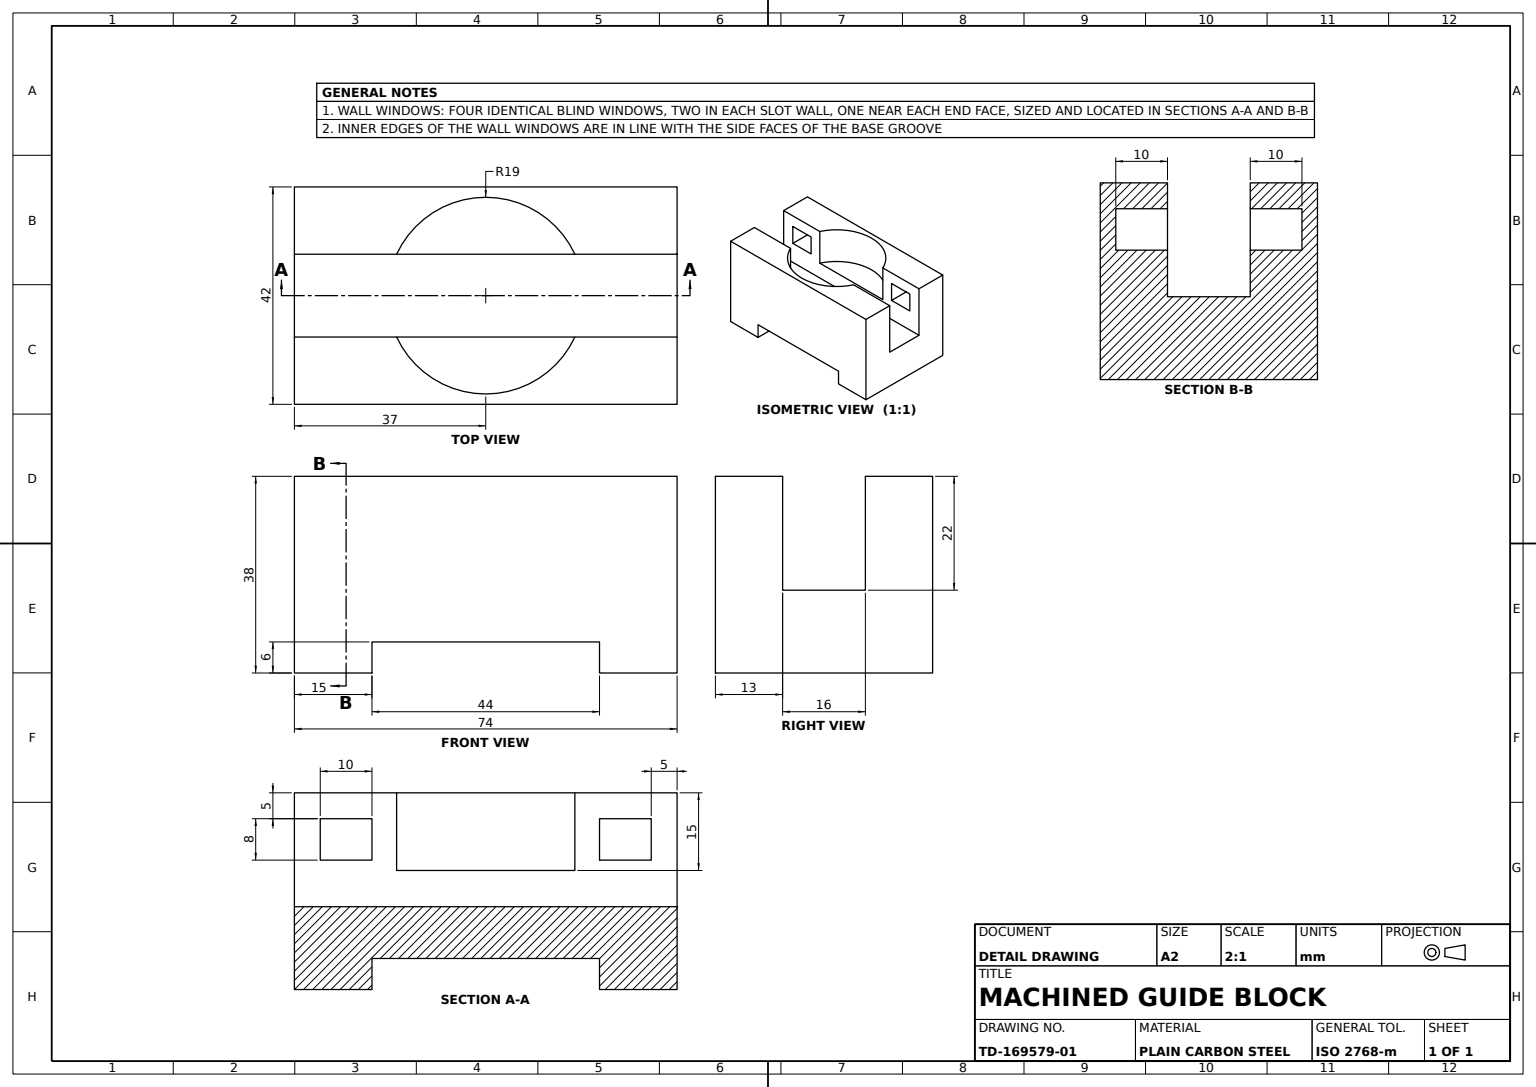
SolidWorks part; units mm, degrees
material "Plain Carbon Steel"
ref_plane "Front Plane" through (0, 0, 0) normal (0, 0, 1) x (1, 0, 0)
ref_plane "Top Plane" through (0, 0, 0) normal (0, 1, 0) x (1, 0, 0)
ref_plane "Right Plane" through (0, 0, 0) normal (1, 0, 0) x (0, 0, -1)
sketch "Block Profile Sketch" plane through (0, 0, 0) normal (0, 0, 1) x (1, 0, 0)
  line L0 (-21, 0) -> (21, 0)
  line L1 (21, 0) -> (21, 38)
  line L2 (21, 38) -> (8, 38)
  line L3 (8, 38) -> (8, 16)
  line L4 (8, 16) -> (-8, 16)
  line L5 (-8, 16) -> (-8, 38)
  line L6 (-8, 38) -> (-21, 38)
  line L7 (-21, 38) -> (-21, 0)
  point P4 (0, 0)
  dimension "D1" = 42
  dimension "D2" = 38
  dimension "D3" = 13
  dimension "D4" = 22
  dimension "D5" = 16
  dimension "D6" = 13
  dimension "D7" = 22
extrude "Block Body" add sketch "Block Profile Sketch" against normal blind 74
sketch "Base Groove Sketch" plane through (21, 0, 0) normal (1, 0, 0) x (0, 0, -1)
  line L1 (74, 0) -> (0, 0) construction
  line L2 (15, 0) -> (15, 6)
  line L3 (15, 6) -> (59, 6)
  line L4 (59, 6) -> (59, 0)
  line L6 (74, 0) -> (74, 38) construction
  line L8 (15, 0) -> (59, 0)
  dimension "D1" = 44
  dimension "D3" = 6
  dimension "D4" = 15
extrude "Base Groove 44x6" cut sketch "Base Groove Sketch" against normal through all
sketch "Bore Sketch" plane through (0, 38, 0) normal (0, 1, 0) x (1, 0, 0)
  line L0 (21, 74) -> (21, 0) construction
  line L1 (21, 0) -> (8, 0) construction
  circle A0 centre (0, 37) radius 19
  dimension "D1" = 38
  dimension "D2" = 21
  dimension "D3" = 37
extrude "Bore Ø38" cut sketch "Bore Sketch" against normal blind 15
sketch "Wall Windows A Sketch" plane through (-8, 0, 0) normal (1, 0, 0) x (0, 0, -1)
  line L0 (0, 0) -> (0, 38) construction
  line L1 (5, 25) -> (15, 25)
  line L2 (5, 25) -> (5, 33)
  line L3 (5, 33) -> (15, 33)
  line L4 (15, 25) -> (15, 33)
  line L5 (74, 38) -> (0, 38) construction
  line L6 (19.7663, 38) -> (19.7663, 23) construction
  line L7 (59, 25) -> (59, 33)
  line L8 (69, 33) -> (59, 33)
  line L9 (69, 25) -> (69, 33)
  line L10 (69, 25) -> (59, 25)
  dimension "D1" = 10
  dimension "D2" = 8
  dimension "D3" = 5
  dimension "D4" = 5
  dimension "D5" = 39.2337
extrude "Wall Windows A 10x8" cut sketch "Wall Windows A Sketch" against normal blind 10
sketch "Wall Windows B Sketch" plane through (8, 0, 0) normal (-1, 0, 0) x (0, 0, 1)
  line L0 (-74, 38) -> (0, 38) construction
  line L1 (-69, 25) -> (-59, 25)
  line L2 (-69, 25) -> (-69, 33)
  line L3 (-69, 33) -> (-59, 33)
  line L4 (-59, 25) -> (-59, 33)
  line L5 (-74, 38) -> (-74, 0) construction
  line L6 (-59, 6) -> (-15, 6) construction
  line L7 (-37, 6) -> (-37, 37.7205) construction
  line L8 (-15, 25) -> (-15, 33)
  line L9 (-5, 33) -> (-15, 33)
  line L10 (-5, 25) -> (-5, 33)
  line L11 (-5, 25) -> (-15, 25)
  dimension "D1" = 10
  dimension "D2" = 8
  dimension "D3" = 5
  dimension "D4" = 5
extrude "Wall Windows B 10x8" cut sketch "Wall Windows B Sketch" against normal blind 10
